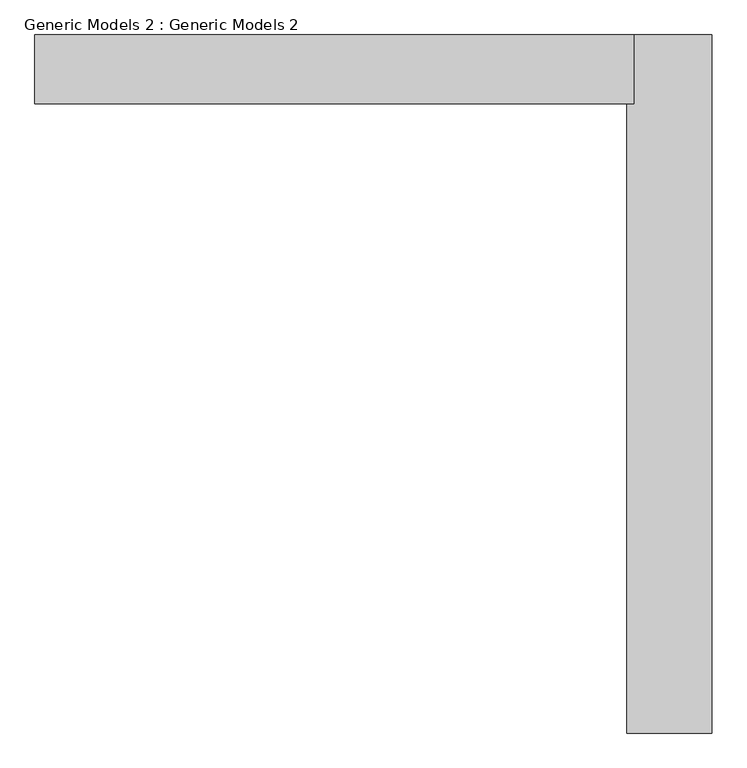
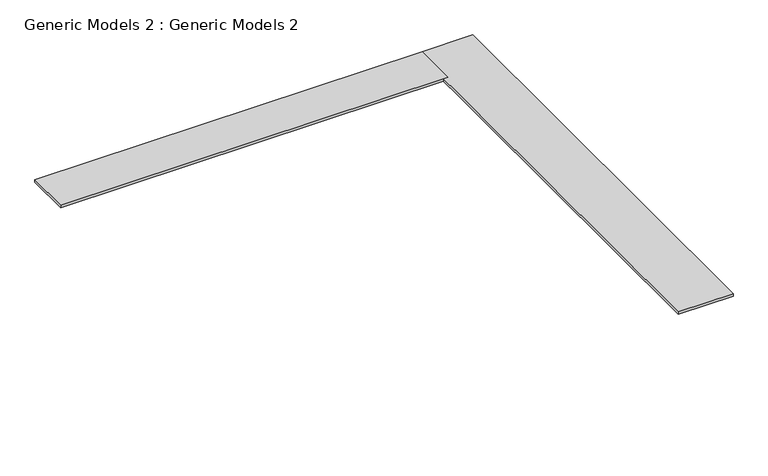
"""IFC4 building model written with IfcOpenShell, lengths in millimetres: proxy geometry, Generic Models 2 : Generic Models 2."""

from ifc_helpers import new_model, si_unit, frame, origin, place, context, project, spatial, polyline, outline, extrude, source, transform, mapped, element, save


def generic_models_2_generic_models_2_aa56fe40(model_context):
    return source(origin(), model_context, "Body", "SweptSolid", [
        extrude(outline(polyline([(13633.4058463, 18209.1799341), (-4095.7941537, 18209.1799341), (-4095.7941537, 20249.067514), (13633.4058463, 20249.067514), (13633.4058463, 18209.1799341)])), frame((0.0, 0.0, -76.2), z_axis=(0.0, 0.0, 1.0), x_axis=(1.0, 0.0, 0.0)), (0.0, 0.0, 1.0), 119.0013059),
        extrude(outline(polyline([(15944.8058463, 20249.067514), (15944.8058463, -401.132486), (13430.2058463, -401.132486), (13430.2058463, 20249.067514), (15944.8058463, 20249.067514)])), frame((0.0, 0.0, -76.2), z_axis=(0.0, 0.0, 1.0), x_axis=(1.0, 0.0, 0.0)), (0.0, 0.0, 1.0), 116.5333435),
    ])


if __name__ == "__main__":
    model = new_model("IFC4")
    model_context = context("Model", 3, world=origin())
    ifc_project = project(units=[si_unit("LENGTHUNIT", "METRE", prefix="MILLI")], contexts=[model_context])
    site = spatial("IfcSite", under=ifc_project)
    building = spatial("IfcBuilding", under=site)
    placement = place(None, origin())
    generic_models_2_generic_models_2_shape = generic_models_2_generic_models_2_aa56fe40(model_context)
    element("IfcBuildingElementProxy", 1, Name="Generic Models 2 : Generic Models 2", ObjectType="Generic Models 2 : Generic Models 2", at=placement, inside=building, context=model_context, shape_type="MappedRepresentation", body=[
        mapped(generic_models_2_generic_models_2_shape, transform((0.0, 0.0, 0.0), x_axis=(1.0, 0.0, 0.0), y_axis=(0.0, 1.0, 0.0), z_axis=(0.0, 0.0, 1.0))),
    ])
    save(model, "model.ifc")
